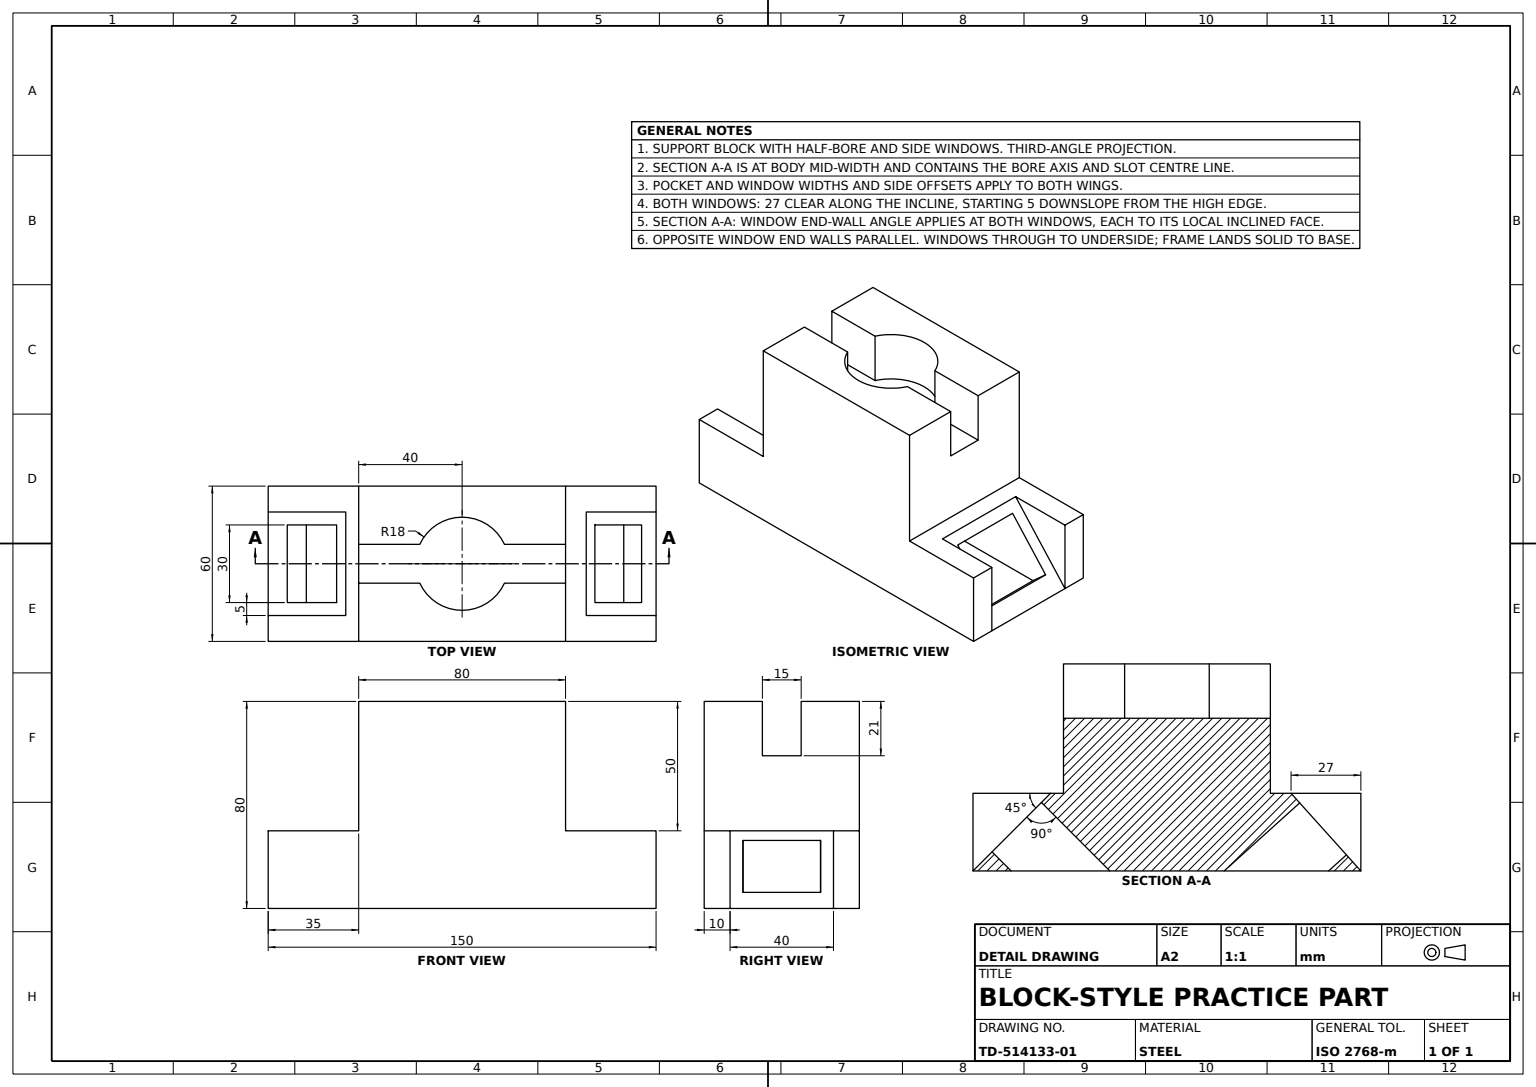
from build123d import *

# Parameters (mm, degrees)
BASE_BLOCK_DEPTH           = 60
BORE_SKETCH_R              = 18
HALF_BORE_CUT_DEPTH        = 21
TOP_SLOT_SKETCH_W          = 80
TOP_SLOT_SKETCH_H          = 15
TOP_SLOT_CUT_DEPTH         = 21
SIDE_POCKET_A_SKETCH_W     = 27
SIDE_POCKET_A_SKETCH_H     = 40
SIDE_POCKET_A_DEPTH        = 40
FRAME_INFILL_A_DEPTH       = 40
TRIANGLE_WINDOW_A_SKETCH_W = 30
TRIANGLE_WINDOW_A_SKETCH_H = 27
TRIANGLE_WINDOW_A_DEPTH    = 40
SIDE_POCKET_B_SKETCH_W     = 30
SIDE_POCKET_B_SKETCH_H     = 40
SIDE_POCKET_B_DEPTH        = 40
FRAME_INFILL_B_DEPTH       = 40
TRIANGLE_WINDOW_B_SKETCH_W = 30
TRIANGLE_WINDOW_B_SKETCH_H = 27
TRIANGLE_WINDOW_B_DEPTH    = 40


with BuildPart() as part:
    # Base Profile Sketch → Base Block (new body)
    with BuildSketch(Plane.XY):
        Polygon((-47.817836812, 0), (102.182163188, 0), (102.182163188, 30), (67.182163188, 30), (67.182163188, 80), (-12.817836812, 80), (-12.817836812, 30), (-47.817836812, 30), align=None)
    extrude(amount=-BASE_BLOCK_DEPTH)

    # Bore Sketch → Half Bore Cut (cut)
    with BuildSketch(Plane(origin=(0, 80, 0), x_dir=(1, 0, 0), z_dir=(0, 1, 0))):
        with Locations(Location((27.182163188, 30, 0), (0, 0, 180))):
            Circle(BORE_SKETCH_R)
    extrude(amount=-HALF_BORE_CUT_DEPTH, mode=Mode.SUBTRACT)

    # Top Slot Sketch → Top Slot Cut (cut)
    with BuildSketch(Plane(origin=(0, 80, 0), x_dir=(1, 0, 0), z_dir=(0, 1, 0))):
        with Locations((27.182163188, 30)):
            Rectangle(TOP_SLOT_SKETCH_W, TOP_SLOT_SKETCH_H)
    extrude(amount=-TOP_SLOT_CUT_DEPTH, mode=Mode.SUBTRACT)

    # Side Pocket A Sketch → Side Pocket A (cut)
    with BuildSketch(Plane(origin=(0, 30, 0), x_dir=(1, 0, 0), z_dir=(0, 1, 0))):
        with Locations((88.682163188, 30)):
            Rectangle(SIDE_POCKET_A_SKETCH_W, SIDE_POCKET_A_SKETCH_H)
    extrude(amount=-SIDE_POCKET_A_DEPTH, mode=Mode.SUBTRACT)

    # Frame Infill A Sketch → Frame Infill A (add)
    with BuildSketch(Plane.XY.offset(-50)):
        Polygon((75.182163188, 30), (102.182163188, 0), (75.182163188, 0), align=None)
    extrude(amount=FRAME_INFILL_A_DEPTH)

    # Triangle Window A Sketch → Triangle Window A (cut)
    with BuildSketch(Plane(origin=(56.454233805, 50.808810425, 0), x_dir=(0, 0, -1), z_dir=(0.7432941462471663, 0.6689647316224498, 0))):
        with Locations((30, -46.495391232)):
            Rectangle(TRIANGLE_WINDOW_A_SKETCH_W, TRIANGLE_WINDOW_A_SKETCH_H)
    extrude(amount=-TRIANGLE_WINDOW_A_DEPTH, mode=Mode.SUBTRACT)

    # Side Pocket B Sketch → Side Pocket B (cut)
    with BuildSketch(Plane(origin=(0, 30, 0), x_dir=(1, 0, 0), z_dir=(0, 1, 0))):
        with Locations((-32.817836812, 30)):
            Rectangle(SIDE_POCKET_B_SKETCH_W, SIDE_POCKET_B_SKETCH_H)
    extrude(amount=-SIDE_POCKET_B_DEPTH, mode=Mode.SUBTRACT)

    # Frame Infill B Sketch → Frame Infill B (add)
    with BuildSketch(Plane.XY.offset(-50)):
        Polygon((-47.817836812, 0), (-17.817836812, 30), (-17.817836812, 0), align=None)
    extrude(amount=FRAME_INFILL_B_DEPTH)

    # Triangle Window B Sketch → Triangle Window B (cut)
    with BuildSketch(Plane(origin=(-23.908918406, 23.908918406, 0), x_dir=(0, 0, 1), z_dir=(-0.7071067811865476, 0.7071067811865476, 0))):
        with Locations((-30, -9.8859098)):
            Rectangle(TRIANGLE_WINDOW_B_SKETCH_W, TRIANGLE_WINDOW_B_SKETCH_H)
    extrude(amount=-TRIANGLE_WINDOW_B_DEPTH, mode=Mode.SUBTRACT)


solid = part.part
